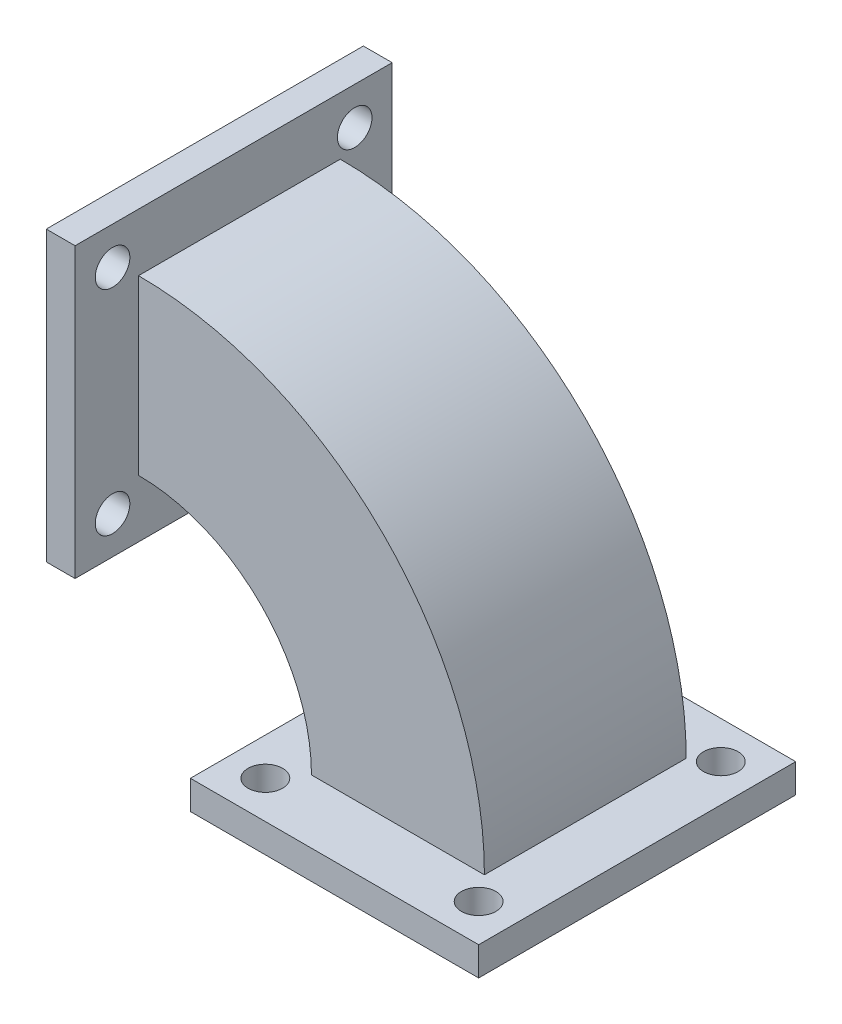
ISO-10303-21;
HEADER;
FILE_DESCRIPTION(('STEP AP214'),'2;1');
FILE_NAME('part.step','',(''),(''),'','','');
FILE_SCHEMA(('AUTOMOTIVE_DESIGN { 1 0 10303 214 1 1 1 1 }'));
ENDSEC;
DATA;
#1=APPLICATION_CONTEXT('core data for automotive mechanical design processes');
#2=APPLICATION_PROTOCOL_DEFINITION('international standard','automotive_design',2000,#1);
#3=PRODUCT_CONTEXT('',#1,'mechanical');
#4=PRODUCT('Part','Part','',(#3));
#5=PRODUCT_RELATED_PRODUCT_CATEGORY('part','',(#4));
#6=PRODUCT_DEFINITION_FORMATION('','',#4);
#7=PRODUCT_DEFINITION_CONTEXT('part definition',#1,'design');
#8=PRODUCT_DEFINITION('design','',#6,#7);
#9=PRODUCT_DEFINITION_SHAPE('','',#8);
#10=(LENGTH_UNIT() NAMED_UNIT(*) SI_UNIT(.MILLI.,.METRE.));
#11=(NAMED_UNIT(*) PLANE_ANGLE_UNIT() SI_UNIT($,.RADIAN.));
#12=(NAMED_UNIT(*) SI_UNIT($,.STERADIAN.) SOLID_ANGLE_UNIT());
#13=UNCERTAINTY_MEASURE_WITH_UNIT(LENGTH_MEASURE(1.E-05),#10,'distance_accuracy_value','');
#14=(GEOMETRIC_REPRESENTATION_CONTEXT(3) GLOBAL_UNCERTAINTY_ASSIGNED_CONTEXT((#13)) GLOBAL_UNIT_ASSIGNED_CONTEXT((#10,
#11,#12)) REPRESENTATION_CONTEXT('',''));
#15=CARTESIAN_POINT('',(0.,0.,0.));
#16=DIRECTION('',(0.,0.,1.));
#17=DIRECTION('',(1.,0.,0.));
#18=AXIS2_PLACEMENT_3D('',#15,#16,#17);
#19=CARTESIAN_POINT('',(0.,0.,55.));
#20=DIRECTION('',(0.,-1.,0.));
#21=DIRECTION('',(0.,0.,-1.));
#22=AXIS2_PLACEMENT_3D('',#19,#20,#21);
#23=PLANE('',#22);
#24=DIRECTION('',(-1.,0.,0.));
#25=VECTOR('',#24,1.);
#26=CARTESIAN_POINT('',(57.,0.,11.));
#27=LINE('',#26,#25);
#28=CARTESIAN_POINT('',(57.,0.,11.));
#29=VERTEX_POINT('',#28);
#30=CARTESIAN_POINT('',(33.,0.,11.));
#31=VERTEX_POINT('',#30);
#32=EDGE_CURVE('E390',#29,#31,#27,.T.);
#33=ORIENTED_EDGE('',*,*,#32,.T.);
#34=DIRECTION('',(0.,0.,1.));
#35=VECTOR('',#34,1.);
#36=CARTESIAN_POINT('',(33.,0.,11.));
#37=LINE('',#36,#35);
#38=CARTESIAN_POINT('',(33.,0.,13.));
#39=VERTEX_POINT('',#38);
#40=EDGE_CURVE('E376',#31,#39,#37,.T.);
#41=ORIENTED_EDGE('',*,*,#40,.T.);
#42=DIRECTION('',(-1.,0.,0.));
#43=VECTOR('',#42,1.);
#44=CARTESIAN_POINT('',(33.,0.,13.));
#45=LINE('',#44,#43);
#46=CARTESIAN_POINT('',(57.,0.,13.));
#47=VERTEX_POINT('',#46);
#48=EDGE_CURVE('E450',#47,#39,#45,.T.);
#49=ORIENTED_EDGE('',*,*,#48,.F.);
#50=DIRECTION('',(0.,0.,1.));
#51=VECTOR('',#50,1.);
#52=CARTESIAN_POINT('',(57.,0.,11.));
#53=LINE('',#52,#51);
#54=EDGE_CURVE('E393',#29,#47,#53,.T.);
#55=ORIENTED_EDGE('',*,*,#54,.F.);
#56=EDGE_LOOP('',(#33,#41,#49,#55));
#57=FACE_BOUND('',#56,.T.);
#58=ADVANCED_FACE('F227',(#57),#23,.F.);
#59=CARTESIAN_POINT('',(0.,0.,55.));
#60=DIRECTION('',(1.,0.,0.));
#61=DIRECTION('',(0.,0.,-1.));
#62=AXIS2_PLACEMENT_3D('',#59,#60,#61);
#63=PLANE('',#62);
#64=DIRECTION('',(0.,0.,1.));
#65=VECTOR('',#64,1.);
#66=CARTESIAN_POINT('',(0.,33.,11.));
#67=LINE('',#66,#65);
#68=CARTESIAN_POINT('',(0.,33.,11.));
#69=VERTEX_POINT('',#68);
#70=CARTESIAN_POINT('',(0.,33.,13.));
#71=VERTEX_POINT('',#70);
#72=EDGE_CURVE('E386',#69,#71,#67,.T.);
#73=ORIENTED_EDGE('',*,*,#72,.F.);
#74=DIRECTION('',(0.,1.,0.));
#75=VECTOR('',#74,1.);
#76=CARTESIAN_POINT('',(0.,57.,11.));
#77=LINE('',#76,#75);
#78=CARTESIAN_POINT('',(0.,57.,11.));
#79=VERTEX_POINT('',#78);
#80=EDGE_CURVE('E249',#69,#79,#77,.T.);
#81=ORIENTED_EDGE('',*,*,#80,.T.);
#82=DIRECTION('',(0.,0.,1.));
#83=VECTOR('',#82,1.);
#84=CARTESIAN_POINT('',(0.,57.,11.));
#85=LINE('',#84,#83);
#86=CARTESIAN_POINT('',(0.,57.,13.));
#87=VERTEX_POINT('',#86);
#88=EDGE_CURVE('E413',#79,#87,#85,.T.);
#89=ORIENTED_EDGE('',*,*,#88,.T.);
#90=DIRECTION('',(0.,1.,0.));
#91=VECTOR('',#90,1.);
#92=CARTESIAN_POINT('',(0.,57.,13.));
#93=LINE('',#92,#91);
#94=EDGE_CURVE('E429',#71,#87,#93,.T.);
#95=ORIENTED_EDGE('',*,*,#94,.F.);
#96=EDGE_LOOP('',(#73,#81,#89,#95));
#97=FACE_BOUND('',#96,.T.);
#98=ADVANCED_FACE('F587',(#97),#63,.T.);
#99=CARTESIAN_POINT('',(0.,0.,55.));
#100=DIRECTION('',(0.,0.,-1.));
#101=DIRECTION('',(-1.,0.,0.));
#102=AXIS2_PLACEMENT_3D('',#99,#100,#101);
#103=CYLINDRICAL_SURFACE('',#102,57.);
#104=ORIENTED_EDGE('',*,*,#88,.F.);
#105=CARTESIAN_POINT('',(0.,0.,11.));
#106=DIRECTION('',(0.,0.,-1.));
#107=DIRECTION('',(-1.,0.,0.));
#108=AXIS2_PLACEMENT_3D('',#105,#106,#107);
#109=CIRCLE('',#108,57.);
#110=EDGE_CURVE('E245',#79,#29,#109,.T.);
#111=ORIENTED_EDGE('',*,*,#110,.T.);
#112=ORIENTED_EDGE('',*,*,#54,.T.);
#113=DIRECTION('',(0.,0.,-1.));
#114=VECTOR('',#113,1.);
#115=CARTESIAN_POINT('',(57.,0.,55.));
#116=LINE('',#115,#114);
#117=CARTESIAN_POINT('',(57.,0.,42.));
#118=VERTEX_POINT('',#117);
#119=EDGE_CURVE('E12',#118,#47,#116,.T.);
#120=ORIENTED_EDGE('',*,*,#119,.F.);
#121=CARTESIAN_POINT('',(0.,0.,42.));
#122=DIRECTION('',(0.,0.,1.));
#123=DIRECTION('',(1.,0.,0.));
#124=AXIS2_PLACEMENT_3D('',#121,#122,#123);
#125=CIRCLE('',#124,57.);
#126=CARTESIAN_POINT('',(0.,57.,42.));
#127=VERTEX_POINT('',#126);
#128=EDGE_CURVE('E411',#127,#118,#125,.F.);
#129=ORIENTED_EDGE('',*,*,#128,.F.);
#130=DIRECTION('',(0.,0.,-1.));
#131=VECTOR('',#130,1.);
#132=CARTESIAN_POINT('',(0.,57.,55.));
#133=LINE('',#132,#131);
#134=EDGE_CURVE('E518',#127,#87,#133,.T.);
#135=ORIENTED_EDGE('',*,*,#134,.T.);
#136=EDGE_LOOP('',(#104,#111,#112,#120,#129,#135));
#137=FACE_BOUND('',#136,.T.);
#138=ADVANCED_FACE('F230',(#137),#103,.F.);
#139=CARTESIAN_POINT('',(0.,0.,55.));
#140=DIRECTION('',(0.,0.,-1.));
#141=DIRECTION('',(-1.,0.,0.));
#142=AXIS2_PLACEMENT_3D('',#139,#140,#141);
#143=CYLINDRICAL_SURFACE('',#142,33.);
#144=CARTESIAN_POINT('',(0.,0.,11.));
#145=DIRECTION('',(0.,0.,1.));
#146=DIRECTION('',(-1.,0.,0.));
#147=AXIS2_PLACEMENT_3D('',#144,#145,#146);
#148=CIRCLE('',#147,33.);
#149=EDGE_CURVE('E379',#31,#69,#148,.T.);
#150=ORIENTED_EDGE('',*,*,#149,.T.);
#151=ORIENTED_EDGE('',*,*,#72,.T.);
#152=DIRECTION('',(0.,0.,-1.));
#153=VECTOR('',#152,1.);
#154=CARTESIAN_POINT('',(0.,33.,55.));
#155=LINE('',#154,#153);
#156=CARTESIAN_POINT('',(0.,33.,42.));
#157=VERTEX_POINT('',#156);
#158=EDGE_CURVE('E495',#157,#71,#155,.T.);
#159=ORIENTED_EDGE('',*,*,#158,.F.);
#160=CARTESIAN_POINT('',(0.,0.,42.));
#161=DIRECTION('',(0.,0.,1.));
#162=DIRECTION('',(1.,0.,0.));
#163=AXIS2_PLACEMENT_3D('',#160,#161,#162);
#164=CIRCLE('',#163,33.);
#165=CARTESIAN_POINT('',(33.,0.,42.));
#166=VERTEX_POINT('',#165);
#167=EDGE_CURVE('E412',#166,#157,#164,.T.);
#168=ORIENTED_EDGE('',*,*,#167,.F.);
#169=DIRECTION('',(0.,0.,-1.));
#170=VECTOR('',#169,1.);
#171=CARTESIAN_POINT('',(33.,0.,55.));
#172=LINE('',#171,#170);
#173=EDGE_CURVE('E385',#166,#39,#172,.T.);
#174=ORIENTED_EDGE('',*,*,#173,.T.);
#175=ORIENTED_EDGE('',*,*,#40,.F.);
#176=EDGE_LOOP('',(#150,#151,#159,#168,#174,#175));
#177=FACE_BOUND('',#176,.T.);
#178=ADVANCED_FACE('F377',(#177),#143,.T.);
#179=CARTESIAN_POINT('',(26.5,0.,6.5));
#180=DIRECTION('',(0.,-1.,0.));
#181=DIRECTION('',(0.,0.,-1.));
#182=AXIS2_PLACEMENT_3D('',#179,#180,#181);
#183=CIRCLE('',#182,3.);
#184=CARTESIAN_POINT('',(26.5,0.,3.5));
#185=VERTEX_POINT('',#184);
#186=EDGE_CURVE('E624',#185,#185,#183,.T.);
#187=ORIENTED_EDGE('',*,*,#186,.T.);
#188=EDGE_LOOP('',(#187));
#189=FACE_BOUND('',#188,.T.);
#190=CARTESIAN_POINT('',(63.5,0.,6.5));
#191=DIRECTION('',(0.,-1.,0.));
#192=DIRECTION('',(0.,0.,-1.));
#193=AXIS2_PLACEMENT_3D('',#190,#191,#192);
#194=CIRCLE('',#193,3.00000000000001);
#195=CARTESIAN_POINT('',(63.5,0.,3.49999999999999));
#196=VERTEX_POINT('',#195);
#197=EDGE_CURVE('E629',#196,#196,#194,.T.);
#198=ORIENTED_EDGE('',*,*,#197,.T.);
#199=EDGE_LOOP('',(#198));
#200=FACE_BOUND('',#199,.T.);
#201=CARTESIAN_POINT('',(63.5,0.,48.5));
#202=DIRECTION('',(0.,-1.,0.));
#203=DIRECTION('',(0.,0.,-1.));
#204=AXIS2_PLACEMENT_3D('',#201,#202,#203);
#205=CIRCLE('',#204,3.00000000000001);
#206=CARTESIAN_POINT('',(63.5,0.,45.5));
#207=VERTEX_POINT('',#206);
#208=EDGE_CURVE('E616',#207,#207,#205,.T.);
#209=ORIENTED_EDGE('',*,*,#208,.T.);
#210=EDGE_LOOP('',(#209));
#211=FACE_BOUND('',#210,.T.);
#212=CARTESIAN_POINT('',(26.5,0.,48.5));
#213=DIRECTION('',(0.,-1.,0.));
#214=DIRECTION('',(0.,0.,-1.));
#215=AXIS2_PLACEMENT_3D('',#212,#213,#214);
#216=CIRCLE('',#215,3.);
#217=CARTESIAN_POINT('',(26.5,0.,45.5));
#218=VERTEX_POINT('',#217);
#219=EDGE_CURVE('E601',#218,#218,#216,.T.);
#220=ORIENTED_EDGE('',*,*,#219,.T.);
#221=EDGE_LOOP('',(#220));
#222=FACE_BOUND('',#221,.T.);
#223=DIRECTION('',(-1.,0.,0.));
#224=VECTOR('',#223,1.);
#225=CARTESIAN_POINT('',(0.,0.,0.));
#226=LINE('',#225,#224);
#227=CARTESIAN_POINT('',(70.,0.,0.));
#228=VERTEX_POINT('',#227);
#229=CARTESIAN_POINT('',(20.,0.,0.));
#230=VERTEX_POINT('',#229);
#231=EDGE_CURVE('E522',#228,#230,#226,.T.);
#232=ORIENTED_EDGE('',*,*,#231,.T.);
#233=DIRECTION('',(0.,0.,-1.));
#234=VECTOR('',#233,1.);
#235=CARTESIAN_POINT('',(20.,0.,55.));
#236=LINE('',#235,#234);
#237=CARTESIAN_POINT('',(20.,0.,55.));
#238=VERTEX_POINT('',#237);
#239=EDGE_CURVE('E473',#238,#230,#236,.T.);
#240=ORIENTED_EDGE('',*,*,#239,.F.);
#241=DIRECTION('',(-1.,0.,0.));
#242=VECTOR('',#241,1.);
#243=CARTESIAN_POINT('',(0.,0.,55.));
#244=LINE('',#243,#242);
#245=CARTESIAN_POINT('',(70.,0.,55.));
#246=VERTEX_POINT('',#245);
#247=EDGE_CURVE('E508',#246,#238,#244,.T.);
#248=ORIENTED_EDGE('',*,*,#247,.F.);
#249=DIRECTION('',(0.,0.,-1.));
#250=VECTOR('',#249,1.);
#251=CARTESIAN_POINT('',(70.,0.,55.));
#252=LINE('',#251,#250);
#253=EDGE_CURVE('E541',#246,#228,#252,.T.);
#254=ORIENTED_EDGE('',*,*,#253,.T.);
#255=EDGE_LOOP('',(#232,#240,#248,#254));
#256=FACE_BOUND('',#255,.T.);
#257=DIRECTION('',(0.,0.,-1.));
#258=VECTOR('',#257,1.);
#259=CARTESIAN_POINT('',(30.,0.,55.));
#260=LINE('',#259,#258);
#261=CARTESIAN_POINT('',(30.,0.,44.));
#262=VERTEX_POINT('',#261);
#263=CARTESIAN_POINT('',(30.,0.,9.));
#264=VERTEX_POINT('',#263);
#265=EDGE_CURVE('E479',#262,#264,#260,.T.);
#266=ORIENTED_EDGE('',*,*,#265,.T.);
#267=DIRECTION('',(-1.,0.,0.));
#268=VECTOR('',#267,1.);
#269=CARTESIAN_POINT('',(0.,0.,9.));
#270=LINE('',#269,#268);
#271=CARTESIAN_POINT('',(60.,0.,9.));
#272=VERTEX_POINT('',#271);
#273=EDGE_CURVE('E405',#272,#264,#270,.T.);
#274=ORIENTED_EDGE('',*,*,#273,.F.);
#275=DIRECTION('',(0.,0.,-1.));
#276=VECTOR('',#275,1.);
#277=CARTESIAN_POINT('',(60.,0.,55.));
#278=LINE('',#277,#276);
#279=CARTESIAN_POINT('',(60.,0.,44.));
#280=VERTEX_POINT('',#279);
#281=EDGE_CURVE('E542',#280,#272,#278,.T.);
#282=ORIENTED_EDGE('',*,*,#281,.F.);
#283=DIRECTION('',(1.,0.,0.));
#284=VECTOR('',#283,1.);
#285=CARTESIAN_POINT('',(0.,0.,44.));
#286=LINE('',#285,#284);
#287=EDGE_CURVE('E419',#262,#280,#286,.T.);
#288=ORIENTED_EDGE('',*,*,#287,.F.);
#289=EDGE_LOOP('',(#266,#274,#282,#288));
#290=FACE_BOUND('',#289,.T.);
#291=ADVANCED_FACE('F638',(#189,#200,#211,#222,#256,#290),#23,.F.);
#292=CARTESIAN_POINT('',(0.,26.5,6.5));
#293=DIRECTION('',(-1.,0.,0.));
#294=DIRECTION('',(0.,0.,1.));
#295=AXIS2_PLACEMENT_3D('',#292,#293,#294);
#296=CIRCLE('',#295,3.);
#297=CARTESIAN_POINT('',(0.,26.5,9.5));
#298=VERTEX_POINT('',#297);
#299=EDGE_CURVE('E598',#298,#298,#296,.T.);
#300=ORIENTED_EDGE('',*,*,#299,.T.);
#301=EDGE_LOOP('',(#300));
#302=FACE_BOUND('',#301,.T.);
#303=CARTESIAN_POINT('',(0.,26.5,48.5));
#304=DIRECTION('',(-1.,0.,0.));
#305=DIRECTION('',(0.,0.,1.));
#306=AXIS2_PLACEMENT_3D('',#303,#304,#305);
#307=CIRCLE('',#306,3.);
#308=CARTESIAN_POINT('',(0.,26.5,51.5));
#309=VERTEX_POINT('',#308);
#310=EDGE_CURVE('E609',#309,#309,#307,.T.);
#311=ORIENTED_EDGE('',*,*,#310,.T.);
#312=EDGE_LOOP('',(#311));
#313=FACE_BOUND('',#312,.T.);
#314=CARTESIAN_POINT('',(0.,63.5,48.5));
#315=DIRECTION('',(-1.,0.,0.));
#316=DIRECTION('',(0.,0.,1.));
#317=AXIS2_PLACEMENT_3D('',#314,#315,#316);
#318=CIRCLE('',#317,3.);
#319=CARTESIAN_POINT('',(0.,63.5,51.5));
#320=VERTEX_POINT('',#319);
#321=EDGE_CURVE('E594',#320,#320,#318,.T.);
#322=ORIENTED_EDGE('',*,*,#321,.T.);
#323=EDGE_LOOP('',(#322));
#324=FACE_BOUND('',#323,.T.);
#325=CARTESIAN_POINT('',(0.,63.5,6.5));
#326=DIRECTION('',(-1.,0.,0.));
#327=DIRECTION('',(0.,0.,1.));
#328=AXIS2_PLACEMENT_3D('',#325,#326,#327);
#329=CIRCLE('',#328,3.);
#330=CARTESIAN_POINT('',(0.,63.5,9.5));
#331=VERTEX_POINT('',#330);
#332=EDGE_CURVE('E590',#331,#331,#329,.T.);
#333=ORIENTED_EDGE('',*,*,#332,.T.);
#334=EDGE_LOOP('',(#333));
#335=FACE_BOUND('',#334,.T.);
#336=DIRECTION('',(0.,1.,0.));
#337=VECTOR('',#336,1.);
#338=CARTESIAN_POINT('',(0.,0.,9.));
#339=LINE('',#338,#337);
#340=CARTESIAN_POINT('',(0.,30.,9.));
#341=VERTEX_POINT('',#340);
#342=CARTESIAN_POINT('',(0.,60.,9.));
#343=VERTEX_POINT('',#342);
#344=EDGE_CURVE('E404',#341,#343,#339,.T.);
#345=ORIENTED_EDGE('',*,*,#344,.F.);
#346=DIRECTION('',(0.,0.,-1.));
#347=VECTOR('',#346,1.);
#348=CARTESIAN_POINT('',(0.,30.,55.));
#349=LINE('',#348,#347);
#350=CARTESIAN_POINT('',(0.,30.,44.));
#351=VERTEX_POINT('',#350);
#352=EDGE_CURVE('E476',#351,#341,#349,.T.);
#353=ORIENTED_EDGE('',*,*,#352,.F.);
#354=DIRECTION('',(0.,-1.,0.));
#355=VECTOR('',#354,1.);
#356=CARTESIAN_POINT('',(0.,0.,44.));
#357=LINE('',#356,#355);
#358=CARTESIAN_POINT('',(0.,60.,44.));
#359=VERTEX_POINT('',#358);
#360=EDGE_CURVE('E428',#359,#351,#357,.T.);
#361=ORIENTED_EDGE('',*,*,#360,.F.);
#362=DIRECTION('',(0.,0.,-1.));
#363=VECTOR('',#362,1.);
#364=CARTESIAN_POINT('',(0.,60.,55.));
#365=LINE('',#364,#363);
#366=EDGE_CURVE('E543',#359,#343,#365,.T.);
#367=ORIENTED_EDGE('',*,*,#366,.T.);
#368=EDGE_LOOP('',(#345,#353,#361,#367));
#369=FACE_BOUND('',#368,.T.);
#370=DIRECTION('',(0.,0.,-1.));
#371=VECTOR('',#370,1.);
#372=CARTESIAN_POINT('',(0.,20.,55.));
#373=LINE('',#372,#371);
#374=CARTESIAN_POINT('',(0.,20.,55.));
#375=VERTEX_POINT('',#374);
#376=CARTESIAN_POINT('',(0.,20.,0.));
#377=VERTEX_POINT('',#376);
#378=EDGE_CURVE('E482',#375,#377,#373,.T.);
#379=ORIENTED_EDGE('',*,*,#378,.T.);
#380=DIRECTION('',(0.,-1.,0.));
#381=VECTOR('',#380,1.);
#382=CARTESIAN_POINT('',(0.,0.,0.));
#383=LINE('',#382,#381);
#384=CARTESIAN_POINT('',(0.,70.,0.));
#385=VERTEX_POINT('',#384);
#386=EDGE_CURVE('E521',#385,#377,#383,.T.);
#387=ORIENTED_EDGE('',*,*,#386,.F.);
#388=DIRECTION('',(0.,0.,-1.));
#389=VECTOR('',#388,1.);
#390=CARTESIAN_POINT('',(0.,70.,55.));
#391=LINE('',#390,#389);
#392=CARTESIAN_POINT('',(0.,70.,55.));
#393=VERTEX_POINT('',#392);
#394=EDGE_CURVE('E538',#393,#385,#391,.T.);
#395=ORIENTED_EDGE('',*,*,#394,.F.);
#396=DIRECTION('',(0.,-1.,0.));
#397=VECTOR('',#396,1.);
#398=CARTESIAN_POINT('',(0.,0.,55.));
#399=LINE('',#398,#397);
#400=EDGE_CURVE('E512',#393,#375,#399,.T.);
#401=ORIENTED_EDGE('',*,*,#400,.T.);
#402=EDGE_LOOP('',(#379,#387,#395,#401));
#403=FACE_BOUND('',#402,.T.);
#404=ADVANCED_FACE('F680',(#302,#313,#324,#335,#369,#403),#63,.T.);
#405=CARTESIAN_POINT('',(0.,0.,55.));
#406=DIRECTION('',(0.,0.,-1.));
#407=DIRECTION('',(-1.,0.,0.));
#408=AXIS2_PLACEMENT_3D('',#405,#406,#407);
#409=CYLINDRICAL_SURFACE('',#408,60.);
#410=ORIENTED_EDGE('',*,*,#281,.T.);
#411=CARTESIAN_POINT('',(0.,0.,9.));
#412=DIRECTION('',(0.,0.,-1.));
#413=DIRECTION('',(-1.,0.,0.));
#414=AXIS2_PLACEMENT_3D('',#411,#412,#413);
#415=CIRCLE('',#414,60.);
#416=EDGE_CURVE('E387',#343,#272,#415,.T.);
#417=ORIENTED_EDGE('',*,*,#416,.F.);
#418=ORIENTED_EDGE('',*,*,#366,.F.);
#419=CARTESIAN_POINT('',(0.,0.,44.));
#420=DIRECTION('',(0.,0.,1.));
#421=DIRECTION('',(1.,0.,0.));
#422=AXIS2_PLACEMENT_3D('',#419,#420,#421);
#423=CIRCLE('',#422,60.);
#424=EDGE_CURVE('E421',#280,#359,#423,.T.);
#425=ORIENTED_EDGE('',*,*,#424,.F.);
#426=EDGE_LOOP('',(#410,#417,#418,#425));
#427=FACE_BOUND('',#426,.T.);
#428=ADVANCED_FACE('F688',(#427),#409,.T.);
#429=CARTESIAN_POINT('',(0.,0.,55.));
#430=DIRECTION('',(0.,0.,-1.));
#431=DIRECTION('',(-1.,0.,0.));
#432=AXIS2_PLACEMENT_3D('',#429,#430,#431);
#433=CYLINDRICAL_SURFACE('',#432,30.);
#434=ORIENTED_EDGE('',*,*,#352,.T.);
#435=CARTESIAN_POINT('',(0.,0.,9.));
#436=DIRECTION('',(0.,0.,-1.));
#437=DIRECTION('',(-1.,0.,0.));
#438=AXIS2_PLACEMENT_3D('',#435,#436,#437);
#439=CIRCLE('',#438,30.);
#440=EDGE_CURVE('E396',#341,#264,#439,.T.);
#441=ORIENTED_EDGE('',*,*,#440,.T.);
#442=ORIENTED_EDGE('',*,*,#265,.F.);
#443=CARTESIAN_POINT('',(0.,0.,44.));
#444=DIRECTION('',(0.,0.,1.));
#445=DIRECTION('',(1.,0.,0.));
#446=AXIS2_PLACEMENT_3D('',#443,#444,#445);
#447=CIRCLE('',#446,30.);
#448=EDGE_CURVE('E420',#351,#262,#447,.F.);
#449=ORIENTED_EDGE('',*,*,#448,.F.);
#450=EDGE_LOOP('',(#434,#441,#442,#449));
#451=FACE_BOUND('',#450,.T.);
#452=ADVANCED_FACE('F853',(#451),#433,.F.);
#453=CARTESIAN_POINT('',(0.,0.,0.));
#454=DIRECTION('',(0.,0.,1.));
#455=DIRECTION('',(1.,0.,0.));
#456=AXIS2_PLACEMENT_3D('',#453,#454,#455);
#457=PLANE('',#456);
#458=ORIENTED_EDGE('',*,*,#386,.T.);
#459=DIRECTION('',(1.,0.,0.));
#460=VECTOR('',#459,1.);
#461=CARTESIAN_POINT('',(0.,20.,0.));
#462=LINE('',#461,#460);
#463=CARTESIAN_POINT('',(-5.,20.,0.));
#464=VERTEX_POINT('',#463);
#465=EDGE_CURVE('E453',#464,#377,#462,.T.);
#466=ORIENTED_EDGE('',*,*,#465,.F.);
#467=DIRECTION('',(0.,1.,0.));
#468=VECTOR('',#467,1.);
#469=CARTESIAN_POINT('',(-5.,0.,0.));
#470=LINE('',#469,#468);
#471=CARTESIAN_POINT('',(-5.,70.,0.));
#472=VERTEX_POINT('',#471);
#473=EDGE_CURVE('E510',#464,#472,#470,.T.);
#474=ORIENTED_EDGE('',*,*,#473,.T.);
#475=DIRECTION('',(1.,0.,0.));
#476=VECTOR('',#475,1.);
#477=CARTESIAN_POINT('',(0.,70.,0.));
#478=LINE('',#477,#476);
#479=EDGE_CURVE('E530',#472,#385,#478,.T.);
#480=ORIENTED_EDGE('',*,*,#479,.T.);
#481=EDGE_LOOP('',(#458,#466,#474,#480));
#482=FACE_BOUND('',#481,.T.);
#483=ADVANCED_FACE('F856',(#482),#457,.F.);
#484=DIRECTION('',(0.,1.,0.));
#485=VECTOR('',#484,1.);
#486=CARTESIAN_POINT('',(20.,0.,0.));
#487=LINE('',#486,#485);
#488=CARTESIAN_POINT('',(20.,-5.,0.));
#489=VERTEX_POINT('',#488);
#490=EDGE_CURVE('E456',#489,#230,#487,.T.);
#491=ORIENTED_EDGE('',*,*,#490,.T.);
#492=ORIENTED_EDGE('',*,*,#231,.F.);
#493=DIRECTION('',(0.,1.,0.));
#494=VECTOR('',#493,1.);
#495=CARTESIAN_POINT('',(70.,0.,0.));
#496=LINE('',#495,#494);
#497=CARTESIAN_POINT('',(70.,-5.,0.));
#498=VERTEX_POINT('',#497);
#499=EDGE_CURVE('E523',#498,#228,#496,.T.);
#500=ORIENTED_EDGE('',*,*,#499,.F.);
#501=DIRECTION('',(1.,0.,0.));
#502=VECTOR('',#501,1.);
#503=CARTESIAN_POINT('',(0.,-5.,0.));
#504=LINE('',#503,#502);
#505=EDGE_CURVE('E501',#489,#498,#504,.T.);
#506=ORIENTED_EDGE('',*,*,#505,.F.);
#507=EDGE_LOOP('',(#491,#492,#500,#506));
#508=FACE_BOUND('',#507,.T.);
#509=ADVANCED_FACE('F948',(#508),#457,.F.);
#510=CARTESIAN_POINT('',(0.,0.,55.));
#511=DIRECTION('',(0.,0.,1.));
#512=DIRECTION('',(1.,0.,0.));
#513=AXIS2_PLACEMENT_3D('',#510,#511,#512);
#514=PLANE('',#513);
#515=DIRECTION('',(1.,0.,0.));
#516=VECTOR('',#515,1.);
#517=CARTESIAN_POINT('',(0.,20.,55.));
#518=LINE('',#517,#516);
#519=CARTESIAN_POINT('',(-5.,20.,55.));
#520=VERTEX_POINT('',#519);
#521=EDGE_CURVE('E458',#520,#375,#518,.T.);
#522=ORIENTED_EDGE('',*,*,#521,.T.);
#523=ORIENTED_EDGE('',*,*,#400,.F.);
#524=DIRECTION('',(1.,0.,0.));
#525=VECTOR('',#524,1.);
#526=CARTESIAN_POINT('',(0.,70.,55.));
#527=LINE('',#526,#525);
#528=CARTESIAN_POINT('',(-5.,70.,55.));
#529=VERTEX_POINT('',#528);
#530=EDGE_CURVE('E514',#529,#393,#527,.T.);
#531=ORIENTED_EDGE('',*,*,#530,.F.);
#532=DIRECTION('',(0.,1.,0.));
#533=VECTOR('',#532,1.);
#534=CARTESIAN_POINT('',(-5.,0.,55.));
#535=LINE('',#534,#533);
#536=EDGE_CURVE('E516',#520,#529,#535,.T.);
#537=ORIENTED_EDGE('',*,*,#536,.F.);
#538=EDGE_LOOP('',(#522,#523,#531,#537));
#539=FACE_BOUND('',#538,.T.);
#540=ADVANCED_FACE('F850',(#539),#514,.T.);
#541=CARTESIAN_POINT('',(57.,0.,55.));
#542=DIRECTION('',(1.,0.,0.));
#543=DIRECTION('',(0.,0.,-1.));
#544=AXIS2_PLACEMENT_3D('',#541,#542,#543);
#545=PLANE('',#544);
#546=ORIENTED_EDGE('',*,*,#119,.T.);
#547=DIRECTION('',(0.,-1.,0.));
#548=VECTOR('',#547,1.);
#549=CARTESIAN_POINT('',(57.,0.,13.));
#550=LINE('',#549,#548);
#551=CARTESIAN_POINT('',(57.,-5.,13.));
#552=VERTEX_POINT('',#551);
#553=EDGE_CURVE('E446',#47,#552,#550,.T.);
#554=ORIENTED_EDGE('',*,*,#553,.T.);
#555=DIRECTION('',(0.,0.,-1.));
#556=VECTOR('',#555,1.);
#557=CARTESIAN_POINT('',(57.,-5.,55.));
#558=LINE('',#557,#556);
#559=CARTESIAN_POINT('',(57.,-5.,42.));
#560=VERTEX_POINT('',#559);
#561=EDGE_CURVE('E232',#560,#552,#558,.T.);
#562=ORIENTED_EDGE('',*,*,#561,.F.);
#563=DIRECTION('',(0.,-1.,0.));
#564=VECTOR('',#563,1.);
#565=CARTESIAN_POINT('',(57.,0.,42.));
#566=LINE('',#565,#564);
#567=EDGE_CURVE('E497',#118,#560,#566,.T.);
#568=ORIENTED_EDGE('',*,*,#567,.F.);
#569=EDGE_LOOP('',(#546,#554,#562,#568));
#570=FACE_BOUND('',#569,.T.);
#571=ADVANCED_FACE('F571',(#570),#545,.F.);
#572=CARTESIAN_POINT('',(0.,-5.,55.));
#573=DIRECTION('',(0.,1.,0.));
#574=DIRECTION('',(0.,0.,1.));
#575=AXIS2_PLACEMENT_3D('',#572,#573,#574);
#576=PLANE('',#575);
#577=CARTESIAN_POINT('',(26.5,-5.,6.5));
#578=DIRECTION('',(0.,-1.,0.));
#579=DIRECTION('',(0.,0.,-1.));
#580=AXIS2_PLACEMENT_3D('',#577,#578,#579);
#581=CIRCLE('',#580,3.);
#582=CARTESIAN_POINT('',(26.5,-5.,3.5));
#583=VERTEX_POINT('',#582);
#584=EDGE_CURVE('E623',#583,#583,#581,.T.);
#585=ORIENTED_EDGE('',*,*,#584,.F.);
#586=EDGE_LOOP('',(#585));
#587=FACE_BOUND('',#586,.T.);
#588=CARTESIAN_POINT('',(63.5,-5.,6.5));
#589=DIRECTION('',(0.,-1.,0.));
#590=DIRECTION('',(0.,0.,-1.));
#591=AXIS2_PLACEMENT_3D('',#588,#589,#590);
#592=CIRCLE('',#591,3.00000000000001);
#593=CARTESIAN_POINT('',(63.5,-5.,3.49999999999999));
#594=VERTEX_POINT('',#593);
#595=EDGE_CURVE('E630',#594,#594,#592,.T.);
#596=ORIENTED_EDGE('',*,*,#595,.F.);
#597=EDGE_LOOP('',(#596));
#598=FACE_BOUND('',#597,.T.);
#599=CARTESIAN_POINT('',(63.5,-5.,48.5));
#600=DIRECTION('',(0.,-1.,0.));
#601=DIRECTION('',(0.,0.,-1.));
#602=AXIS2_PLACEMENT_3D('',#599,#600,#601);
#603=CIRCLE('',#602,3.00000000000001);
#604=CARTESIAN_POINT('',(63.5,-5.,45.5));
#605=VERTEX_POINT('',#604);
#606=EDGE_CURVE('E633',#605,#605,#603,.T.);
#607=ORIENTED_EDGE('',*,*,#606,.F.);
#608=EDGE_LOOP('',(#607));
#609=FACE_BOUND('',#608,.T.);
#610=CARTESIAN_POINT('',(26.5,-5.,48.5));
#611=DIRECTION('',(0.,-1.,0.));
#612=DIRECTION('',(0.,0.,-1.));
#613=AXIS2_PLACEMENT_3D('',#610,#611,#612);
#614=CIRCLE('',#613,3.);
#615=CARTESIAN_POINT('',(26.5,-5.,45.5));
#616=VERTEX_POINT('',#615);
#617=EDGE_CURVE('E614',#616,#616,#614,.T.);
#618=ORIENTED_EDGE('',*,*,#617,.F.);
#619=EDGE_LOOP('',(#618));
#620=FACE_BOUND('',#619,.T.);
#621=ORIENTED_EDGE('',*,*,#561,.T.);
#622=DIRECTION('',(-1.,0.,0.));
#623=VECTOR('',#622,1.);
#624=CARTESIAN_POINT('',(33.,-5.,13.));
#625=LINE('',#624,#623);
#626=CARTESIAN_POINT('',(33.,-5.,13.));
#627=VERTEX_POINT('',#626);
#628=EDGE_CURVE('E444',#552,#627,#625,.T.);
#629=ORIENTED_EDGE('',*,*,#628,.T.);
#630=DIRECTION('',(0.,0.,-1.));
#631=VECTOR('',#630,1.);
#632=CARTESIAN_POINT('',(33.,-5.,55.));
#633=LINE('',#632,#631);
#634=CARTESIAN_POINT('',(33.,-5.,42.));
#635=VERTEX_POINT('',#634);
#636=EDGE_CURVE('E466',#635,#627,#633,.T.);
#637=ORIENTED_EDGE('',*,*,#636,.F.);
#638=DIRECTION('',(1.,0.,0.));
#639=VECTOR('',#638,1.);
#640=CARTESIAN_POINT('',(33.,-5.,42.));
#641=LINE('',#640,#639);
#642=EDGE_CURVE('E492',#635,#560,#641,.T.);
#643=ORIENTED_EDGE('',*,*,#642,.T.);
#644=EDGE_LOOP('',(#621,#629,#637,#643));
#645=FACE_BOUND('',#644,.T.);
#646=ORIENTED_EDGE('',*,*,#505,.T.);
#647=DIRECTION('',(0.,0.,-1.));
#648=VECTOR('',#647,1.);
#649=CARTESIAN_POINT('',(70.,-5.,55.));
#650=LINE('',#649,#648);
#651=CARTESIAN_POINT('',(70.,-5.,55.));
#652=VERTEX_POINT('',#651);
#653=EDGE_CURVE('E547',#652,#498,#650,.T.);
#654=ORIENTED_EDGE('',*,*,#653,.F.);
#655=DIRECTION('',(1.,0.,0.));
#656=VECTOR('',#655,1.);
#657=CARTESIAN_POINT('',(0.,-5.,55.));
#658=LINE('',#657,#656);
#659=CARTESIAN_POINT('',(20.,-5.,55.));
#660=VERTEX_POINT('',#659);
#661=EDGE_CURVE('E502',#660,#652,#658,.T.);
#662=ORIENTED_EDGE('',*,*,#661,.F.);
#663=DIRECTION('',(0.,0.,-1.));
#664=VECTOR('',#663,1.);
#665=CARTESIAN_POINT('',(20.,-5.,55.));
#666=LINE('',#665,#664);
#667=EDGE_CURVE('E471',#660,#489,#666,.T.);
#668=ORIENTED_EDGE('',*,*,#667,.T.);
#669=EDGE_LOOP('',(#646,#654,#662,#668));
#670=FACE_BOUND('',#669,.T.);
#671=ADVANCED_FACE('F555',(#587,#598,#609,#620,#645,#670),#576,.F.);
#672=CARTESIAN_POINT('',(70.,0.,55.));
#673=DIRECTION('',(-1.,0.,0.));
#674=DIRECTION('',(0.,0.,1.));
#675=AXIS2_PLACEMENT_3D('',#672,#673,#674);
#676=PLANE('',#675);
#677=ORIENTED_EDGE('',*,*,#499,.T.);
#678=ORIENTED_EDGE('',*,*,#253,.F.);
#679=DIRECTION('',(0.,1.,0.));
#680=VECTOR('',#679,1.);
#681=CARTESIAN_POINT('',(70.,0.,55.));
#682=LINE('',#681,#680);
#683=EDGE_CURVE('E506',#652,#246,#682,.T.);
#684=ORIENTED_EDGE('',*,*,#683,.F.);
#685=ORIENTED_EDGE('',*,*,#653,.T.);
#686=EDGE_LOOP('',(#677,#678,#684,#685));
#687=FACE_BOUND('',#686,.T.);
#688=ADVANCED_FACE('F654',(#687),#676,.F.);
#689=CARTESIAN_POINT('',(0.,70.,55.));
#690=DIRECTION('',(0.,1.,0.));
#691=DIRECTION('',(0.,0.,1.));
#692=AXIS2_PLACEMENT_3D('',#689,#690,#691);
#693=PLANE('',#692);
#694=ORIENTED_EDGE('',*,*,#479,.F.);
#695=DIRECTION('',(0.,0.,-1.));
#696=VECTOR('',#695,1.);
#697=CARTESIAN_POINT('',(-5.,70.,55.));
#698=LINE('',#697,#696);
#699=EDGE_CURVE('E537',#529,#472,#698,.T.);
#700=ORIENTED_EDGE('',*,*,#699,.F.);
#701=ORIENTED_EDGE('',*,*,#530,.T.);
#702=ORIENTED_EDGE('',*,*,#394,.T.);
#703=EDGE_LOOP('',(#694,#700,#701,#702));
#704=FACE_BOUND('',#703,.T.);
#705=ADVANCED_FACE('F910',(#704),#693,.T.);
#706=CARTESIAN_POINT('',(-5.,0.,55.));
#707=DIRECTION('',(-1.,0.,0.));
#708=DIRECTION('',(0.,0.,1.));
#709=AXIS2_PLACEMENT_3D('',#706,#707,#708);
#710=PLANE('',#709);
#711=CARTESIAN_POINT('',(-5.,26.5,6.5));
#712=DIRECTION('',(-1.,0.,0.));
#713=DIRECTION('',(0.,0.,1.));
#714=AXIS2_PLACEMENT_3D('',#711,#712,#713);
#715=CIRCLE('',#714,3.);
#716=CARTESIAN_POINT('',(-5.,26.5,9.5));
#717=VERTEX_POINT('',#716);
#718=EDGE_CURVE('E600',#717,#717,#715,.T.);
#719=ORIENTED_EDGE('',*,*,#718,.F.);
#720=EDGE_LOOP('',(#719));
#721=FACE_BOUND('',#720,.T.);
#722=CARTESIAN_POINT('',(-5.,26.5,48.5));
#723=DIRECTION('',(-1.,0.,0.));
#724=DIRECTION('',(0.,0.,1.));
#725=AXIS2_PLACEMENT_3D('',#722,#723,#724);
#726=CIRCLE('',#725,3.);
#727=CARTESIAN_POINT('',(-5.,26.5,51.5));
#728=VERTEX_POINT('',#727);
#729=EDGE_CURVE('E603',#728,#728,#726,.T.);
#730=ORIENTED_EDGE('',*,*,#729,.F.);
#731=EDGE_LOOP('',(#730));
#732=FACE_BOUND('',#731,.T.);
#733=CARTESIAN_POINT('',(-5.,63.5,48.5));
#734=DIRECTION('',(-1.,0.,0.));
#735=DIRECTION('',(0.,0.,1.));
#736=AXIS2_PLACEMENT_3D('',#733,#734,#735);
#737=CIRCLE('',#736,3.);
#738=CARTESIAN_POINT('',(-5.,63.5,51.5));
#739=VERTEX_POINT('',#738);
#740=EDGE_CURVE('E606',#739,#739,#737,.T.);
#741=ORIENTED_EDGE('',*,*,#740,.F.);
#742=EDGE_LOOP('',(#741));
#743=FACE_BOUND('',#742,.T.);
#744=CARTESIAN_POINT('',(-5.,63.5,6.5));
#745=DIRECTION('',(-1.,0.,0.));
#746=DIRECTION('',(0.,0.,1.));
#747=AXIS2_PLACEMENT_3D('',#744,#745,#746);
#748=CIRCLE('',#747,3.);
#749=CARTESIAN_POINT('',(-5.,63.5,9.5));
#750=VERTEX_POINT('',#749);
#751=EDGE_CURVE('E591',#750,#750,#748,.T.);
#752=ORIENTED_EDGE('',*,*,#751,.F.);
#753=EDGE_LOOP('',(#752));
#754=FACE_BOUND('',#753,.T.);
#755=ORIENTED_EDGE('',*,*,#473,.F.);
#756=DIRECTION('',(0.,0.,-1.));
#757=VECTOR('',#756,1.);
#758=CARTESIAN_POINT('',(-5.,20.,55.));
#759=LINE('',#758,#757);
#760=EDGE_CURVE('E488',#520,#464,#759,.T.);
#761=ORIENTED_EDGE('',*,*,#760,.F.);
#762=ORIENTED_EDGE('',*,*,#536,.T.);
#763=ORIENTED_EDGE('',*,*,#699,.T.);
#764=EDGE_LOOP('',(#755,#761,#762,#763));
#765=FACE_BOUND('',#764,.T.);
#766=DIRECTION('',(0.,1.,0.));
#767=VECTOR('',#766,1.);
#768=CARTESIAN_POINT('',(-5.,57.,13.));
#769=LINE('',#768,#767);
#770=CARTESIAN_POINT('',(-5.,33.,13.));
#771=VERTEX_POINT('',#770);
#772=CARTESIAN_POINT('',(-5.,57.,13.));
#773=VERTEX_POINT('',#772);
#774=EDGE_CURVE('E426',#771,#773,#769,.T.);
#775=ORIENTED_EDGE('',*,*,#774,.T.);
#776=DIRECTION('',(0.,0.,-1.));
#777=VECTOR('',#776,1.);
#778=CARTESIAN_POINT('',(-5.,57.,55.));
#779=LINE('',#778,#777);
#780=CARTESIAN_POINT('',(-5.,57.,42.));
#781=VERTEX_POINT('',#780);
#782=EDGE_CURVE('E534',#781,#773,#779,.T.);
#783=ORIENTED_EDGE('',*,*,#782,.F.);
#784=DIRECTION('',(0.,-1.,0.));
#785=VECTOR('',#784,1.);
#786=CARTESIAN_POINT('',(-5.,33.,42.));
#787=LINE('',#786,#785);
#788=CARTESIAN_POINT('',(-5.,33.,42.));
#789=VERTEX_POINT('',#788);
#790=EDGE_CURVE('E440',#781,#789,#787,.T.);
#791=ORIENTED_EDGE('',*,*,#790,.T.);
#792=DIRECTION('',(0.,0.,-1.));
#793=VECTOR('',#792,1.);
#794=CARTESIAN_POINT('',(-5.,33.,55.));
#795=LINE('',#794,#793);
#796=EDGE_CURVE('E490',#789,#771,#795,.T.);
#797=ORIENTED_EDGE('',*,*,#796,.T.);
#798=EDGE_LOOP('',(#775,#783,#791,#797));
#799=FACE_BOUND('',#798,.T.);
#800=ADVANCED_FACE('F578',(#721,#732,#743,#754,#765,#799),#710,.T.);
#801=CARTESIAN_POINT('',(0.,57.,55.));
#802=DIRECTION('',(0.,-1.,0.));
#803=DIRECTION('',(0.,0.,-1.));
#804=AXIS2_PLACEMENT_3D('',#801,#802,#803);
#805=PLANE('',#804);
#806=DIRECTION('',(-1.,0.,0.));
#807=VECTOR('',#806,1.);
#808=CARTESIAN_POINT('',(0.,57.,13.));
#809=LINE('',#808,#807);
#810=EDGE_CURVE('E434',#87,#773,#809,.T.);
#811=ORIENTED_EDGE('',*,*,#810,.F.);
#812=ORIENTED_EDGE('',*,*,#134,.F.);
#813=DIRECTION('',(-1.,0.,0.));
#814=VECTOR('',#813,1.);
#815=CARTESIAN_POINT('',(0.,57.,42.));
#816=LINE('',#815,#814);
#817=EDGE_CURVE('E441',#127,#781,#816,.T.);
#818=ORIENTED_EDGE('',*,*,#817,.T.);
#819=ORIENTED_EDGE('',*,*,#782,.T.);
#820=EDGE_LOOP('',(#811,#812,#818,#819));
#821=FACE_BOUND('',#820,.T.);
#822=ADVANCED_FACE('F574',(#821),#805,.T.);
#823=ORIENTED_EDGE('',*,*,#247,.T.);
#824=DIRECTION('',(0.,1.,0.));
#825=VECTOR('',#824,1.);
#826=CARTESIAN_POINT('',(20.,0.,55.));
#827=LINE('',#826,#825);
#828=EDGE_CURVE('E460',#660,#238,#827,.T.);
#829=ORIENTED_EDGE('',*,*,#828,.F.);
#830=ORIENTED_EDGE('',*,*,#661,.T.);
#831=ORIENTED_EDGE('',*,*,#683,.T.);
#832=EDGE_LOOP('',(#823,#829,#830,#831));
#833=FACE_BOUND('',#832,.T.);
#834=ADVANCED_FACE('F835',(#833),#514,.T.);
#835=CARTESIAN_POINT('',(33.,0.,42.));
#836=DIRECTION('',(0.,0.,-1.));
#837=DIRECTION('',(-1.,0.,0.));
#838=AXIS2_PLACEMENT_3D('',#835,#836,#837);
#839=PLANE('',#838);
#840=ORIENTED_EDGE('',*,*,#642,.F.);
#841=DIRECTION('',(0.,-1.,0.));
#842=VECTOR('',#841,1.);
#843=CARTESIAN_POINT('',(33.,0.,42.));
#844=LINE('',#843,#842);
#845=EDGE_CURVE('E498',#166,#635,#844,.T.);
#846=ORIENTED_EDGE('',*,*,#845,.F.);
#847=ORIENTED_EDGE('',*,*,#167,.T.);
#848=DIRECTION('',(-1.,0.,0.));
#849=VECTOR('',#848,1.);
#850=CARTESIAN_POINT('',(0.,33.,42.));
#851=LINE('',#850,#849);
#852=EDGE_CURVE('E445',#157,#789,#851,.T.);
#853=ORIENTED_EDGE('',*,*,#852,.T.);
#854=ORIENTED_EDGE('',*,*,#790,.F.);
#855=ORIENTED_EDGE('',*,*,#817,.F.);
#856=ORIENTED_EDGE('',*,*,#128,.T.);
#857=ORIENTED_EDGE('',*,*,#567,.T.);
#858=EDGE_LOOP('',(#840,#846,#847,#853,#854,#855,#856,#857));
#859=FACE_BOUND('',#858,.T.);
#860=ADVANCED_FACE('F570',(#859),#839,.T.);
#861=CARTESIAN_POINT('',(0.,33.,55.));
#862=DIRECTION('',(0.,-1.,0.));
#863=DIRECTION('',(0.,0.,-1.));
#864=AXIS2_PLACEMENT_3D('',#861,#862,#863);
#865=PLANE('',#864);
#866=ORIENTED_EDGE('',*,*,#158,.T.);
#867=DIRECTION('',(-1.,0.,0.));
#868=VECTOR('',#867,1.);
#869=CARTESIAN_POINT('',(0.,33.,13.));
#870=LINE('',#869,#868);
#871=EDGE_CURVE('E435',#71,#771,#870,.T.);
#872=ORIENTED_EDGE('',*,*,#871,.T.);
#873=ORIENTED_EDGE('',*,*,#796,.F.);
#874=ORIENTED_EDGE('',*,*,#852,.F.);
#875=EDGE_LOOP('',(#866,#872,#873,#874));
#876=FACE_BOUND('',#875,.T.);
#877=ADVANCED_FACE('F588',(#876),#865,.F.);
#878=CARTESIAN_POINT('',(0.,20.,55.));
#879=DIRECTION('',(0.,1.,0.));
#880=DIRECTION('',(0.,0.,1.));
#881=AXIS2_PLACEMENT_3D('',#878,#879,#880);
#882=PLANE('',#881);
#883=ORIENTED_EDGE('',*,*,#465,.T.);
#884=ORIENTED_EDGE('',*,*,#378,.F.);
#885=ORIENTED_EDGE('',*,*,#521,.F.);
#886=ORIENTED_EDGE('',*,*,#760,.T.);
#887=EDGE_LOOP('',(#883,#884,#885,#886));
#888=FACE_BOUND('',#887,.T.);
#889=ADVANCED_FACE('F823',(#888),#882,.F.);
#890=CARTESIAN_POINT('',(20.,0.,55.));
#891=DIRECTION('',(-1.,0.,0.));
#892=DIRECTION('',(0.,0.,1.));
#893=AXIS2_PLACEMENT_3D('',#890,#891,#892);
#894=PLANE('',#893);
#895=ORIENTED_EDGE('',*,*,#490,.F.);
#896=ORIENTED_EDGE('',*,*,#667,.F.);
#897=ORIENTED_EDGE('',*,*,#828,.T.);
#898=ORIENTED_EDGE('',*,*,#239,.T.);
#899=EDGE_LOOP('',(#895,#896,#897,#898));
#900=FACE_BOUND('',#899,.T.);
#901=ADVANCED_FACE('F815',(#900),#894,.T.);
#902=CARTESIAN_POINT('',(33.,0.,55.));
#903=DIRECTION('',(1.,0.,0.));
#904=DIRECTION('',(0.,0.,-1.));
#905=AXIS2_PLACEMENT_3D('',#902,#903,#904);
#906=PLANE('',#905);
#907=DIRECTION('',(0.,-1.,0.));
#908=VECTOR('',#907,1.);
#909=CARTESIAN_POINT('',(33.,0.,13.));
#910=LINE('',#909,#908);
#911=EDGE_CURVE('E452',#39,#627,#910,.T.);
#912=ORIENTED_EDGE('',*,*,#911,.F.);
#913=ORIENTED_EDGE('',*,*,#173,.F.);
#914=ORIENTED_EDGE('',*,*,#845,.T.);
#915=ORIENTED_EDGE('',*,*,#636,.T.);
#916=EDGE_LOOP('',(#912,#913,#914,#915));
#917=FACE_BOUND('',#916,.T.);
#918=ADVANCED_FACE('F562',(#917),#906,.T.);
#919=CARTESIAN_POINT('',(33.,0.,13.));
#920=DIRECTION('',(0.,0.,1.));
#921=DIRECTION('',(1.,0.,0.));
#922=AXIS2_PLACEMENT_3D('',#919,#920,#921);
#923=PLANE('',#922);
#924=ORIENTED_EDGE('',*,*,#628,.F.);
#925=ORIENTED_EDGE('',*,*,#553,.F.);
#926=ORIENTED_EDGE('',*,*,#48,.T.);
#927=ORIENTED_EDGE('',*,*,#911,.T.);
#928=EDGE_LOOP('',(#924,#925,#926,#927));
#929=FACE_BOUND('',#928,.T.);
#930=ADVANCED_FACE('F561',(#929),#923,.T.);
#931=CARTESIAN_POINT('',(0.,57.,13.));
#932=DIRECTION('',(0.,0.,1.));
#933=DIRECTION('',(1.,0.,0.));
#934=AXIS2_PLACEMENT_3D('',#931,#932,#933);
#935=PLANE('',#934);
#936=ORIENTED_EDGE('',*,*,#774,.F.);
#937=ORIENTED_EDGE('',*,*,#871,.F.);
#938=ORIENTED_EDGE('',*,*,#94,.T.);
#939=ORIENTED_EDGE('',*,*,#810,.T.);
#940=EDGE_LOOP('',(#936,#937,#938,#939));
#941=FACE_BOUND('',#940,.T.);
#942=ADVANCED_FACE('F584',(#941),#935,.T.);
#943=CARTESIAN_POINT('',(0.,0.,44.));
#944=DIRECTION('',(0.,0.,1.));
#945=DIRECTION('',(1.,0.,0.));
#946=AXIS2_PLACEMENT_3D('',#943,#944,#945);
#947=PLANE('',#946);
#948=ORIENTED_EDGE('',*,*,#287,.T.);
#949=ORIENTED_EDGE('',*,*,#424,.T.);
#950=ORIENTED_EDGE('',*,*,#360,.T.);
#951=ORIENTED_EDGE('',*,*,#448,.T.);
#952=EDGE_LOOP('',(#948,#949,#950,#951));
#953=FACE_BOUND('',#952,.T.);
#954=ADVANCED_FACE('F773',(#953),#947,.T.);
#955=CARTESIAN_POINT('',(0.,0.,9.));
#956=DIRECTION('',(0.,0.,-1.));
#957=DIRECTION('',(-1.,0.,0.));
#958=AXIS2_PLACEMENT_3D('',#955,#956,#957);
#959=PLANE('',#958);
#960=ORIENTED_EDGE('',*,*,#273,.T.);
#961=ORIENTED_EDGE('',*,*,#440,.F.);
#962=ORIENTED_EDGE('',*,*,#344,.T.);
#963=ORIENTED_EDGE('',*,*,#416,.T.);
#964=EDGE_LOOP('',(#960,#961,#962,#963));
#965=FACE_BOUND('',#964,.T.);
#966=ADVANCED_FACE('F764',(#965),#959,.T.);
#967=CARTESIAN_POINT('',(0.,0.,11.));
#968=DIRECTION('',(0.,0.,-1.));
#969=DIRECTION('',(-1.,0.,0.));
#970=AXIS2_PLACEMENT_3D('',#967,#968,#969);
#971=PLANE('',#970);
#972=ORIENTED_EDGE('',*,*,#110,.F.);
#973=ORIENTED_EDGE('',*,*,#80,.F.);
#974=ORIENTED_EDGE('',*,*,#149,.F.);
#975=ORIENTED_EDGE('',*,*,#32,.F.);
#976=EDGE_LOOP('',(#972,#973,#974,#975));
#977=FACE_BOUND('',#976,.T.);
#978=ADVANCED_FACE('F395',(#977),#971,.F.);
#979=CARTESIAN_POINT('',(0.,63.5,6.5));
#980=DIRECTION('',(-1.,0.,0.));
#981=DIRECTION('',(0.,0.,1.));
#982=AXIS2_PLACEMENT_3D('',#979,#980,#981);
#983=CYLINDRICAL_SURFACE('',#982,3.);
#984=ORIENTED_EDGE('',*,*,#332,.F.);
#985=EDGE_LOOP('',(#984));
#986=FACE_BOUND('',#985,.T.);
#987=ORIENTED_EDGE('',*,*,#751,.T.);
#988=EDGE_LOOP('',(#987));
#989=FACE_BOUND('',#988,.T.);
#990=ADVANCED_FACE('F748',(#986,#989),#983,.F.);
#991=CARTESIAN_POINT('',(0.,63.5,48.5));
#992=DIRECTION('',(-1.,0.,0.));
#993=DIRECTION('',(0.,0.,1.));
#994=AXIS2_PLACEMENT_3D('',#991,#992,#993);
#995=CYLINDRICAL_SURFACE('',#994,3.);
#996=ORIENTED_EDGE('',*,*,#321,.F.);
#997=EDGE_LOOP('',(#996));
#998=FACE_BOUND('',#997,.T.);
#999=ORIENTED_EDGE('',*,*,#740,.T.);
#1000=EDGE_LOOP('',(#999));
#1001=FACE_BOUND('',#1000,.T.);
#1002=ADVANCED_FACE('F738',(#998,#1001),#995,.F.);
#1003=CARTESIAN_POINT('',(0.,26.5,48.5));
#1004=DIRECTION('',(-1.,0.,0.));
#1005=DIRECTION('',(0.,0.,1.));
#1006=AXIS2_PLACEMENT_3D('',#1003,#1004,#1005);
#1007=CYLINDRICAL_SURFACE('',#1006,3.);
#1008=ORIENTED_EDGE('',*,*,#310,.F.);
#1009=EDGE_LOOP('',(#1008));
#1010=FACE_BOUND('',#1009,.T.);
#1011=ORIENTED_EDGE('',*,*,#729,.T.);
#1012=EDGE_LOOP('',(#1011));
#1013=FACE_BOUND('',#1012,.T.);
#1014=ADVANCED_FACE('F664',(#1010,#1013),#1007,.F.);
#1015=CARTESIAN_POINT('',(0.,26.5,6.5));
#1016=DIRECTION('',(-1.,0.,0.));
#1017=DIRECTION('',(0.,0.,1.));
#1018=AXIS2_PLACEMENT_3D('',#1015,#1016,#1017);
#1019=CYLINDRICAL_SURFACE('',#1018,3.);
#1020=ORIENTED_EDGE('',*,*,#299,.F.);
#1021=EDGE_LOOP('',(#1020));
#1022=FACE_BOUND('',#1021,.T.);
#1023=ORIENTED_EDGE('',*,*,#718,.T.);
#1024=EDGE_LOOP('',(#1023));
#1025=FACE_BOUND('',#1024,.T.);
#1026=ADVANCED_FACE('F657',(#1022,#1025),#1019,.F.);
#1027=CARTESIAN_POINT('',(26.5,0.,48.5));
#1028=DIRECTION('',(0.,-1.,0.));
#1029=DIRECTION('',(0.,0.,-1.));
#1030=AXIS2_PLACEMENT_3D('',#1027,#1028,#1029);
#1031=CYLINDRICAL_SURFACE('',#1030,3.);
#1032=ORIENTED_EDGE('',*,*,#219,.F.);
#1033=EDGE_LOOP('',(#1032));
#1034=FACE_BOUND('',#1033,.T.);
#1035=ORIENTED_EDGE('',*,*,#617,.T.);
#1036=EDGE_LOOP('',(#1035));
#1037=FACE_BOUND('',#1036,.T.);
#1038=ADVANCED_FACE('F646',(#1034,#1037),#1031,.F.);
#1039=CARTESIAN_POINT('',(63.5,0.,48.5));
#1040=DIRECTION('',(0.,-1.,0.));
#1041=DIRECTION('',(0.,0.,-1.));
#1042=AXIS2_PLACEMENT_3D('',#1039,#1040,#1041);
#1043=CYLINDRICAL_SURFACE('',#1042,3.00000000000001);
#1044=ORIENTED_EDGE('',*,*,#208,.F.);
#1045=EDGE_LOOP('',(#1044));
#1046=FACE_BOUND('',#1045,.T.);
#1047=ORIENTED_EDGE('',*,*,#606,.T.);
#1048=EDGE_LOOP('',(#1047));
#1049=FACE_BOUND('',#1048,.T.);
#1050=ADVANCED_FACE('F645',(#1046,#1049),#1043,.F.);
#1051=CARTESIAN_POINT('',(63.5,0.,6.5));
#1052=DIRECTION('',(0.,-1.,0.));
#1053=DIRECTION('',(0.,0.,-1.));
#1054=AXIS2_PLACEMENT_3D('',#1051,#1052,#1053);
#1055=CYLINDRICAL_SURFACE('',#1054,3.00000000000001);
#1056=ORIENTED_EDGE('',*,*,#197,.F.);
#1057=EDGE_LOOP('',(#1056));
#1058=FACE_BOUND('',#1057,.T.);
#1059=ORIENTED_EDGE('',*,*,#595,.T.);
#1060=EDGE_LOOP('',(#1059));
#1061=FACE_BOUND('',#1060,.T.);
#1062=ADVANCED_FACE('F643',(#1058,#1061),#1055,.F.);
#1063=CARTESIAN_POINT('',(26.5,0.,6.5));
#1064=DIRECTION('',(0.,-1.,0.));
#1065=DIRECTION('',(0.,0.,-1.));
#1066=AXIS2_PLACEMENT_3D('',#1063,#1064,#1065);
#1067=CYLINDRICAL_SURFACE('',#1066,3.);
#1068=ORIENTED_EDGE('',*,*,#186,.F.);
#1069=EDGE_LOOP('',(#1068));
#1070=FACE_BOUND('',#1069,.T.);
#1071=ORIENTED_EDGE('',*,*,#584,.T.);
#1072=EDGE_LOOP('',(#1071));
#1073=FACE_BOUND('',#1072,.T.);
#1074=ADVANCED_FACE('F696',(#1070,#1073),#1067,.F.);
#1075=CLOSED_SHELL('',(#58,#98,#138,#178,#291,#404,#428,#452,#483,#509,#540,#571,#671,#688,#705,
#800,#822,#834,#860,#877,#889,#901,#918,#930,#942,#954,#966,#978,#990,#1002,#1014,#1026,#1038,
#1050,#1062,#1074));
#1076=MANIFOLD_SOLID_BREP('B2',#1075);
#1077=ADVANCED_BREP_SHAPE_REPRESENTATION('',(#18,#1076),#14);
#1078=SHAPE_DEFINITION_REPRESENTATION(#9,#1077);
ENDSEC;
END-ISO-10303-21;
